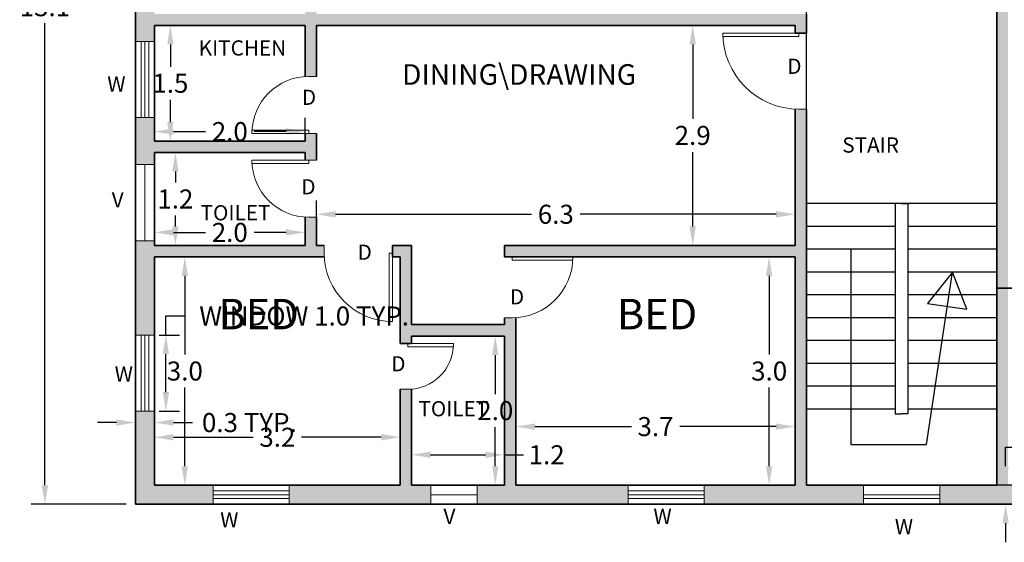
# Model space of a CAD drawing. Units: metres. Extents: x 6.2 to 29.4, y -2.1 to 16.8.
# Tile 1 of 3: x 6.2 to 19.2, y -2.1 to 4.8. Entities that reach past the tile are written whole.
import ezdxf

# ---------------------------------------------------------------- set-up
doc = ezdxf.new("R2010")
doc.units = ezdxf.units.M
doc.header["$MEASUREMENT"] = 0
doc.layers.get('0').update_dxf_attribs({"color": 2})
doc.layers.get('Defpoints').update_dxf_attribs({"color": 3})
for name, color, linetype, lineweight in [('A-ANNO-DIMS', 6, 'Continuous', 13), ('A-ANNO-TEXT', 7, 'Continuous', 18), ('A-AREA-IDEN', 3, 'Continuous', 18), ('A-DOOR', 3, 'Continuous', 18), ('A-FLOR-STRS', 1, 'Continuous', 25), ('A-GLAZ', 4, 'Continuous', 18), ('A-WALL', 7, 'Continuous', 35), ('A-WALL-PATT', 252, 'Continuous', 13)]:
    doc.layers.add(name, color=color, linetype=linetype, lineweight=lineweight)
doc.styles.get("Standard").update_dxf_attribs({"font": 'arial.ttf'})
doc.dimstyles.get("Standard").update_dxf_attribs({"dimtxt": 0.25, "dimasz": 0.25, "dimexe": 0.18, "dimexo": 0.0625, "dimgap": 0.09, "dimtad": 0, "dimtih": 1, "dimtoh": 1, "dimdec": 1, "dimzin": 0, "dimdsep": 46, "dimtxsty": 'Standard', "dimcen": 0.09, "dimadec": 0, "dimazin": 0, "dimtfac": 1, "dimtdec": 1, "dimtofl": 0, "dimtmove": 0, "dimatfit": 3, "dimfxl": 1, "dimtolj": 1, "dimtzin": 0, "dimarcsym": 0})

# ---------------------------------------------------------------- blocks, each defined once
blk = doc.blocks.new('*U2')
for p, q in [((-900, 0), (-900, 100)), ((0, 0), (0, 100))]:
    blk.add_line(p, q)
blk.add_lwpolyline([(0, 0), (0, -900), (-43.75, -900), (-43.75, 0)], close=True)
blk.add_arc((0, 0), 900, 180, 270)
blk = doc.blocks.new('*U3')
for p, q in [((0, 0), (0, -100)), ((600, 0), (600, -100))]:
    blk.add_line(p, q)
blk.add_lwpolyline([(0, 0), (0, 600), (43.75, 600), (43.75, 0)], close=True)
blk.add_arc((0, 0), 600, 0, 90)
blk = doc.blocks.new('*U4')
for p, q in [((-800, 0), (-800, 100)), ((0, 0), (0, 100))]:
    blk.add_line(p, q)
blk.add_lwpolyline([(0, 0), (0, -800), (-43.75, -800), (-43.75, 0)], close=True)
blk.add_arc((0, 0), 800, 180, 270)
blk = doc.blocks.new('*D5')
at = {"layer": 'A-ANNO-DIMS', "color": 0, "lineweight": -2, "transparency": 16777216}
for p, q in [((8.047, 1.673), (8.563, 1.673)), ((8.383, 1.423), (8.383, 0.391)), ((8.383, -1.077), (8.383, -0.045)), ((8.047, -1.327), (8.563, -1.327))]:
    blk.add_line(p, q, dxfattribs=at)
at = {"layer": 'A-ANNO-DIMS', "color": 0, "transparency": 16777216}
for points in [[(8.341, 1.423), (8.424, 1.423), (8.383, 1.673)], [(8.341, -1.077), (8.424, -1.077), (8.383, -1.327)]]:
    blk.add_solid(points, dxfattribs=at)
at = {"layer": 'Defpoints', "color": 0, "transparency": 16777216}
for p in [(7.984, 1.673), (7.984, -1.327), (8.383, -1.327)]:
    blk.add_point(p, dxfattribs=at)
at = {"layer": 'A-ANNO-DIMS', "color": 0, "transparency": 16777216, "insert": (8.383, 0.173), "char_height": 0.25, "attachment_point": 5}
blk.add_mtext('\\A1;3.0', dxfattribs=at)
blk = doc.blocks.new('*D6')
at = {"layer": 'A-ANNO-DIMS', "color": 0, "lineweight": -2, "transparency": 16777216}
for p, q in [((7.984, -1.264), (7.984, -0.517)), ((11.214, -1.264), (11.214, -0.517)), ((8.234, -0.697), (9.283, -0.697)), ((10.964, -0.697), (9.915, -0.697))]:
    blk.add_line(p, q, dxfattribs=at)
at = {"layer": 'A-ANNO-DIMS', "color": 0, "transparency": 16777216}
for points in [[(8.234, -0.655), (8.234, -0.739), (7.984, -0.697)], [(10.964, -0.655), (10.964, -0.739), (11.214, -0.697)]]:
    blk.add_solid(points, dxfattribs=at)
at = {"layer": 'Defpoints', "color": 0, "transparency": 16777216}
for p in [(11.214, -0.697), (7.984, -1.327), (11.214, -1.327)]:
    blk.add_point(p, dxfattribs=at)
at = {"layer": 'A-ANNO-DIMS', "color": 0, "transparency": 16777216, "insert": (9.599, -0.697), "char_height": 0.25, "attachment_point": 5}
blk.add_mtext('\\A1;3.2', dxfattribs=at)
blk = doc.blocks.new('*D7')
at = {"layer": 'A-ANNO-DIMS', "color": 0, "lineweight": -2, "transparency": 16777216}
for p, q in [((12.522, 0.633), (12.283, 0.633)), ((12.463, 0.383), (12.463, -0.129)), ((12.463, -1.077), (12.463, -0.565)), ((12.522, -1.327), (12.283, -1.327))]:
    blk.add_line(p, q, dxfattribs=at)
at = {"layer": 'A-ANNO-DIMS', "color": 0, "transparency": 16777216}
for points in [[(12.421, 0.383), (12.504, 0.383), (12.463, 0.633)], [(12.421, -1.077), (12.504, -1.077), (12.463, -1.327)]]:
    blk.add_solid(points, dxfattribs=at)
at = {"layer": 'Defpoints', "color": 0, "transparency": 16777216}
for p in [(12.584, 0.633), (12.463, -1.327), (12.584, -1.327)]:
    blk.add_point(p, dxfattribs=at)
at = {"layer": 'A-ANNO-DIMS', "color": 0, "transparency": 16777216, "insert": (12.463, -0.347), "char_height": 0.25, "attachment_point": 5}
blk.add_mtext('\\A1;2.0', dxfattribs=at)
blk = doc.blocks.new('*D8')
at = {"layer": 'A-ANNO-DIMS', "color": 0, "lineweight": -2, "transparency": 16777216}
for p, q in [((11.364, -1.264), (11.364, -0.747)), ((12.584, -1.264), (12.584, -0.747)), ((11.614, -0.927), (12.334, -0.927)), ((12.584, -0.927), (12.834, -0.927))]:
    blk.add_line(p, q, dxfattribs=at)
at = {"layer": 'A-ANNO-DIMS', "color": 0, "transparency": 16777216}
for points in [[(11.614, -0.886), (11.614, -0.969), (11.364, -0.927)], [(12.334, -0.886), (12.334, -0.969), (12.584, -0.927)]]:
    blk.add_solid(points, dxfattribs=at)
at = {"layer": 'Defpoints', "color": 0, "transparency": 16777216}
for p in [(12.584, -0.927), (11.364, -1.327), (12.584, -1.327)]:
    blk.add_point(p, dxfattribs=at)
at = {"layer": 'A-ANNO-DIMS', "color": 0, "transparency": 16777216, "insert": (13.139, -0.927), "char_height": 0.25, "attachment_point": 5}
blk.add_mtext('\\A1;1.2', dxfattribs=at)
blk = doc.blocks.new('*D9')
at = {"layer": 'A-ANNO-DIMS', "color": 0, "lineweight": -2, "transparency": 16777216}
for p, q in [((16.342, 1.673), (15.883, 1.673)), ((16.063, 1.423), (16.063, 0.391)), ((16.063, -1.077), (16.063, -0.045)), ((16.342, -1.327), (15.883, -1.327))]:
    blk.add_line(p, q, dxfattribs=at)
at = {"layer": 'A-ANNO-DIMS', "color": 0, "transparency": 16777216}
for points in [[(16.021, 1.423), (16.104, 1.423), (16.063, 1.673)], [(16.021, -1.077), (16.104, -1.077), (16.063, -1.327)]]:
    blk.add_solid(points, dxfattribs=at)
at = {"layer": 'Defpoints', "color": 0, "transparency": 16777216}
for p in [(16.404, 1.673), (16.063, -1.327), (16.404, -1.327)]:
    blk.add_point(p, dxfattribs=at)
at = {"layer": 'A-ANNO-DIMS', "color": 0, "transparency": 16777216, "insert": (16.063, 0.173), "char_height": 0.25, "attachment_point": 5}
blk.add_mtext('\\A1;3.0', dxfattribs=at)
blk = doc.blocks.new('*D10')
at = {"layer": 'A-ANNO-DIMS', "color": 0, "lineweight": -2, "transparency": 16777216}
for p, q in [((12.734, -1.264), (12.734, -0.377)), ((16.404, -1.264), (16.404, -0.377)), ((12.984, -0.557), (14.252, -0.557)), ((16.154, -0.557), (14.887, -0.557))]:
    blk.add_line(p, q, dxfattribs=at)
at = {"layer": 'A-ANNO-DIMS', "color": 0, "transparency": 16777216}
for points in [[(12.984, -0.516), (12.984, -0.599), (12.734, -0.557)], [(16.154, -0.516), (16.154, -0.599), (16.404, -0.557)]]:
    blk.add_solid(points, dxfattribs=at)
at = {"layer": 'Defpoints', "color": 0, "transparency": 16777216}
for p in [(16.404, -0.557), (12.734, -1.327), (16.404, -1.327)]:
    blk.add_point(p, dxfattribs=at)
at = {"layer": 'A-ANNO-DIMS', "color": 0, "transparency": 16777216, "insert": (14.569, -0.557), "char_height": 0.25, "attachment_point": 5}
blk.add_mtext('\\A1;3.7', dxfattribs=at)
blk = doc.blocks.new('*U17')
for p, q in [((-750, 0), (-750, -100)), ((0, 0), (0, -100))]:
    blk.add_line(p, q)
blk.add_lwpolyline([(0, 0), (0, 750), (-43.75, 750), (-43.75, 0)], close=True)
blk.add_arc((0, 0), 750, 90, 180)
blk = doc.blocks.new('*D18')
at = {"layer": 'A-ANNO-DIMS', "color": 0, "lineweight": -2, "transparency": 16777216}
for p, q in [((8.047, 4.713), (8.373, 4.713)), ((8.193, 4.463), (8.193, 4.171)), ((8.193, 3.443), (8.193, 3.735)), ((8.047, 3.193), (8.373, 3.193))]:
    blk.add_line(p, q, dxfattribs=at)
at = {"layer": 'A-ANNO-DIMS', "color": 0, "transparency": 16777216}
for points in [[(8.151, 4.463), (8.234, 4.463), (8.193, 4.713)], [(8.151, 3.443), (8.234, 3.443), (8.193, 3.193)]]:
    blk.add_solid(points, dxfattribs=at)
at = {"layer": 'Defpoints', "color": 0, "transparency": 16777216}
for p in [(7.984, 4.713), (7.984, 3.193), (8.193, 3.193)]:
    blk.add_point(p, dxfattribs=at)
at = {"layer": 'A-ANNO-DIMS', "color": 0, "transparency": 16777216, "insert": (8.193, 3.953), "char_height": 0.25, "attachment_point": 5}
blk.add_mtext('\\A1;1.5', dxfattribs=at)
blk = doc.blocks.new('*D19')
at = {"layer": 'A-ANNO-DIMS', "color": 0, "lineweight": -2, "transparency": 16777216}
for p, q in [((7.984, 3.256), (7.984, 3.498)), ((9.964, 3.256), (9.964, 3.498)), ((8.234, 3.318), (8.655, 3.318)), ((9.714, 3.318), (9.293, 3.318))]:
    blk.add_line(p, q, dxfattribs=at)
at = {"layer": 'A-ANNO-DIMS', "color": 0, "transparency": 16777216}
for points in [[(8.234, 3.36), (8.234, 3.277), (7.984, 3.318)], [(9.714, 3.36), (9.714, 3.277), (9.964, 3.318)]]:
    blk.add_solid(points, dxfattribs=at)
at = {"layer": 'Defpoints', "color": 0, "transparency": 16777216}
for p in [(7.984, 3.318), (7.984, 3.193), (9.964, 3.193)]:
    blk.add_point(p, dxfattribs=at)
at = {"layer": 'A-ANNO-DIMS', "color": 0, "transparency": 16777216, "insert": (8.974, 3.318), "char_height": 0.25, "attachment_point": 5}
blk.add_mtext('\\A1;2.0', dxfattribs=at)
blk = doc.blocks.new('*D20')
at = {"layer": 'A-ANNO-DIMS', "color": 0, "lineweight": -2, "transparency": 16777216}
for p, q in [((8.047, 3.043), (8.439, 3.043)), ((8.259, 2.793), (8.259, 2.649)), ((8.259, 2.073), (8.259, 2.218)), ((8.047, 1.823), (8.439, 1.823))]:
    blk.add_line(p, q, dxfattribs=at)
at = {"layer": 'A-ANNO-DIMS', "color": 0, "transparency": 16777216}
for points in [[(8.217, 2.793), (8.301, 2.793), (8.259, 3.043)], [(8.217, 2.073), (8.301, 2.073), (8.259, 1.823)]]:
    blk.add_solid(points, dxfattribs=at)
at = {"layer": 'Defpoints', "color": 0, "transparency": 16777216}
for p in [(7.984, 3.043), (7.984, 1.823), (8.259, 1.823)]:
    blk.add_point(p, dxfattribs=at)
at = {"layer": 'A-ANNO-DIMS', "color": 0, "transparency": 16777216, "insert": (8.259, 2.433), "char_height": 0.25, "attachment_point": 5}
blk.add_mtext('\\A1;1.2', dxfattribs=at)
blk = doc.blocks.new('*D21')
at = {"layer": 'A-ANNO-DIMS', "color": 0, "lineweight": -2, "transparency": 16777216}
for p, q in [((7.984, 1.886), (7.984, 2.174)), ((9.964, 1.886), (9.964, 2.174)), ((8.234, 1.994), (8.655, 1.994)), ((9.714, 1.994), (9.293, 1.994))]:
    blk.add_line(p, q, dxfattribs=at)
at = {"layer": 'A-ANNO-DIMS', "color": 0, "transparency": 16777216}
for points in [[(8.234, 2.036), (8.234, 1.952), (7.984, 1.994)], [(9.714, 2.036), (9.714, 1.952), (9.964, 1.994)]]:
    blk.add_solid(points, dxfattribs=at)
at = {"layer": 'Defpoints', "color": 0, "transparency": 16777216}
for p in [(7.984, 1.994), (7.984, 1.823), (9.964, 1.823)]:
    blk.add_point(p, dxfattribs=at)
at = {"layer": 'A-ANNO-DIMS', "color": 0, "transparency": 16777216, "insert": (8.974, 1.994), "char_height": 0.25, "attachment_point": 5}
blk.add_mtext('\\A1;2.0', dxfattribs=at)
blk = doc.blocks.new('*U22')
for p, q in [((0, 0), (0, -100)), ((-1000, 0), (-1000, -100))]:
    blk.add_line(p, q)
blk.add_lwpolyline([(0, 0), (0, 1000), (-43.75, 1000), (-43.75, 0)], close=True)
blk.add_arc((0, 0), 1000, 90, 180)
blk = doc.blocks.new('*D23')
at = {"layer": 'A-ANNO-DIMS', "color": 0, "lineweight": -2, "transparency": 16777216}
for p, q in [((14.995, 4.713), (14.878, 4.713)), ((15.058, 4.463), (15.058, 3.486)), ((15.058, 2.073), (15.058, 3.05)), ((14.995, 1.823), (14.878, 1.823))]:
    blk.add_line(p, q, dxfattribs=at)
at = {"layer": 'A-ANNO-DIMS', "color": 0, "transparency": 16777216}
for points in [[(15.016, 4.463), (15.1, 4.463), (15.058, 4.713)], [(15.016, 2.073), (15.1, 2.073), (15.058, 1.823)]]:
    blk.add_solid(points, dxfattribs=at)
at = {"layer": 'Defpoints', "color": 0, "transparency": 16777216}
for p in [(15.058, 4.713), (15.058, 1.823), (15.058, 1.823)]:
    blk.add_point(p, dxfattribs=at)
at = {"layer": 'A-ANNO-DIMS', "color": 0, "transparency": 16777216, "insert": (15.058, 3.268), "char_height": 0.25, "attachment_point": 5}
blk.add_mtext('\\A1;2.9', dxfattribs=at)
blk = doc.blocks.new('*D24')
at = {"layer": 'A-ANNO-DIMS', "color": 0, "lineweight": -2, "transparency": 16777216}
for p, q in [((10.114, 2.071), (10.114, 2.412)), ((16.404, 2.071), (16.404, 2.412)), ((10.364, 2.232), (12.941, 2.232)), ((16.154, 2.232), (13.577, 2.232))]:
    blk.add_line(p, q, dxfattribs=at)
at = {"layer": 'A-ANNO-DIMS', "color": 0, "transparency": 16777216}
for points in [[(10.364, 2.274), (10.364, 2.19), (10.114, 2.232)], [(16.154, 2.274), (16.154, 2.19), (16.404, 2.232)]]:
    blk.add_solid(points, dxfattribs=at)
at = {"layer": 'Defpoints', "color": 0, "transparency": 16777216}
for p in [(16.404, 2.232), (10.114, 2.008), (16.404, 2.008)]:
    blk.add_point(p, dxfattribs=at)
at = {"layer": 'A-ANNO-DIMS', "color": 0, "transparency": 16777216, "insert": (13.259, 2.232), "char_height": 0.25, "attachment_point": 5}
blk.add_mtext('\\A1;6.3', dxfattribs=at)
blk = doc.blocks.new('*D60')
at = {"layer": 'A-ANNO-DIMS', "color": 0, "lineweight": -2, "transparency": 16777216}
for p, q in [((7.611, 11.494), (6.364, 11.494)), ((6.544, 11.244), (6.544, 5.176)), ((6.544, -1.327), (6.544, 4.741)), ((7.611, -1.577), (6.364, -1.577))]:
    blk.add_line(p, q, dxfattribs=at)
at = {"layer": 'A-ANNO-DIMS', "color": 0, "transparency": 16777216}
for points in [[(6.502, 11.244), (6.586, 11.244), (6.544, 11.494)], [(6.502, -1.327), (6.586, -1.327), (6.544, -1.577)]]:
    blk.add_solid(points, dxfattribs=at)
at = {"layer": 'Defpoints', "color": 0, "transparency": 16777216}
for p in [(7.674, 11.494), (6.544, -1.577), (7.674, -1.577)]:
    blk.add_point(p, dxfattribs=at)
at = {"layer": 'A-ANNO-DIMS', "color": 0, "transparency": 16777216, "insert": (6.544, 4.959), "char_height": 0.25, "attachment_point": 5}
blk.add_mtext('\\A1;13.1', dxfattribs=at)
blk = doc.blocks.new('WIN-1000')
for p, q in [((0.075, 1), (0.075, 0)), ((0.125, 1), (0.125, 0)), ((0.175, 1), (0.175, 0))]:
    blk.add_line(p, q)
blk.add_lwpolyline([(0, 1), (0.25, 1), (0.25, 0), (0, 0)], close=True)
blk = doc.blocks.new('VENT-1000')
blk.add_line((0.125, 1), (0.125, 0))
blk.add_lwpolyline([(0, 1), (0.25, 1), (0.25, 0), (0, 0)], close=True)
blk = doc.blocks.new('*D65')
at = {"layer": 'A-ANNO-DIMS', "color": 0, "lineweight": -2, "transparency": 16777216}
for p, q in [((8.134, 0.646), (8.134, 0.896)), ((8.134, 0.896), (8.384, 0.896)), ((8.047, 0.646), (8.314, 0.646)), ((8.134, -0.104), (8.134, 0.396)), ((8.047, -0.354), (8.314, -0.354))]:
    blk.add_line(p, q, dxfattribs=at)
at = {"layer": 'A-ANNO-DIMS', "color": 0, "transparency": 16777216}
for points in [[(8.092, 0.396), (8.176, 0.396), (8.134, 0.646)], [(8.092, -0.104), (8.176, -0.104), (8.134, -0.354)]]:
    blk.add_solid(points, dxfattribs=at)
at = {"layer": 'Defpoints', "color": 0, "transparency": 16777216}
for p in [(7.984, 0.646), (8.134, 0.646), (7.984, -0.354)]:
    blk.add_point(p, dxfattribs=at)
at = {"layer": 'A-ANNO-DIMS', "color": 0, "transparency": 16777216, "insert": (9.951, 0.896), "char_height": 0.25, "attachment_point": 5}
blk.add_mtext('\\A1;WINDOW 1.0 TYP.', dxfattribs=at)
blk = doc.blocks.new('*D66')
at = {"layer": 'A-ANNO-DIMS', "color": 0, "lineweight": -2, "transparency": 16777216}
for p, q in [((7.484, -0.504), (7.234, -0.504)), ((7.734, -0.416), (7.734, -0.684)), ((7.984, -0.416), (7.984, -0.684)), ((8.234, -0.504), (8.484, -0.504))]:
    blk.add_line(p, q, dxfattribs=at)
at = {"layer": 'A-ANNO-DIMS', "color": 0, "transparency": 16777216}
for points in [[(7.484, -0.462), (7.484, -0.545), (7.734, -0.504)], [(8.234, -0.462), (8.234, -0.545), (7.984, -0.504)]]:
    blk.add_solid(points, dxfattribs=at)
at = {"layer": 'Defpoints', "color": 0, "transparency": 16777216}
for p in [(7.734, -0.354), (7.984, -0.354), (7.984, -0.504)]:
    blk.add_point(p, dxfattribs=at)
at = {"layer": 'A-ANNO-DIMS', "color": 0, "transparency": 16777216, "insert": (9.231, -0.504), "char_height": 0.25, "attachment_point": 5}
blk.add_mtext('\\A1;0.3 TYP.', dxfattribs=at)
blk = doc.blocks.new('*D70')
at = {"layer": 'A-ANNO-DIMS', "color": 0, "lineweight": -2, "transparency": 16777216}
for p, q in [((19.17, -1.077), (19.17, -0.827)), ((19.17, -0.827), (19.42, -0.827)), ((19.258, -1.327), (18.99, -1.327)), ((19.258, -1.577), (18.99, -1.577)), ((19.17, -1.827), (19.17, -2.077))]:
    blk.add_line(p, q, dxfattribs=at)
at = {"layer": 'A-ANNO-DIMS', "color": 0, "transparency": 16777216}
for points in [[(19.129, -1.077), (19.212, -1.077), (19.17, -1.327)], [(19.129, -1.827), (19.212, -1.827), (19.17, -1.577)]]:
    blk.add_solid(points, dxfattribs=at)
at = {"layer": 'Defpoints', "color": 0, "transparency": 16777216}
for p in [(19.17, -1.327), (19.32, -1.327), (19.32, -1.577)]:
    blk.add_point(p, dxfattribs=at)
at = {"layer": 'A-ANNO-DIMS', "color": 0, "transparency": 16777216, "insert": (20.167, -0.827), "char_height": 0.25, "attachment_point": 5}
blk.add_mtext('\\A1;0.3 TYP.', dxfattribs=at)
blk = doc.blocks.new('*D71')
at = {"layer": 'A-ANNO-DIMS', "color": 0, "lineweight": -2, "transparency": 16777216}
for p, q in [((16.554, 2.436), (16.554, 15.849)), ((19.054, 2.436), (19.054, 15.849)), ((16.804, 15.669), (17.483, 15.669)), ((18.804, 15.669), (18.125, 15.669))]:
    blk.add_line(p, q, dxfattribs=at)
at = {"layer": 'A-ANNO-DIMS', "color": 0, "transparency": 16777216}
for points in [[(16.804, 15.71), (16.804, 15.627), (16.554, 15.669)], [(18.804, 15.71), (18.804, 15.627), (19.054, 15.669)]]:
    blk.add_solid(points, dxfattribs=at)
at = {"layer": 'Defpoints', "color": 0, "transparency": 16777216}
for p in [(19.054, 15.669), (16.554, 2.373), (19.054, 2.373)]:
    blk.add_point(p, dxfattribs=at)
at = {"layer": 'A-ANNO-DIMS', "color": 0, "transparency": 16777216, "insert": (17.804, 15.669), "char_height": 0.25, "attachment_point": 5}
blk.add_mtext('\\A1;2.5', dxfattribs=at)

msp = doc.modelspace()

# ---------------------------------------------------------------- hatches: boundary and pattern name
at = {"layer": 'A-WALL-PATT'}
h = msp.add_hatch(dxfattribs=at)
h.set_pattern_fill('BRICK', color=256, scale=0.3)
h.paths.add_polyline_path([(26.024, -0.354), (25.774, -0.354), (25.774, -1.327), (24.478, -1.327), (24.478, -1.577), (26.024, -1.577)])
h.paths.add_polyline_path([(26.024, 2.199), (25.774, 2.199), (25.774, 2.123), (24.325, 2.123, -0.063254), (24.344, 1.973), (24.344, 1.873), (25.774, 1.873), (25.774, 0.646), (26.024, 0.646)])
h.paths.add_polyline_path([(26.624, 4.802), (26.374, 4.802), (26.374, 3.493), (23.373, 3.493, -0.013897), (23.374, 3.443), (23.374, 3.343), (23.494, 3.343), (23.494, 2.123), (23.344, 2.123), (23.344, 2.023, -0.03766), (23.333, 1.873), (23.744, 1.873), (23.744, 1.973), (23.744, 2.123), (23.644, 2.123), (23.644, 3.343), (25.774, 3.343), (25.774, 3.199), (26.024, 3.199), (26.024, 3.343), (26.624, 3.343)])
h.paths.add_polyline_path([(26.624, 6.775), (26.374, 6.775), (26.374, 6.693), (24.244, 6.693), (24.244, 7.065, -0.016681), (24.194, 7.063), (24.094, 7.063), (24.094, 6.693), (19.054, 6.693), (19.054, 6.443), (19.154, 6.443), (19.204, 6.443), (19.204, 6.543), (22.224, 6.543), (22.224, 3.343), (22.474, 3.343), (22.474, 3.443), (22.474, 3.493), (22.374, 3.493), (22.374, 6.543), (26.374, 6.543), (26.374, 5.802), (26.624, 5.802)])
h.paths.add_polyline_path([(26.624, 8.282), (26.374, 8.282), (26.374, 8.063), (24.244, 8.063), (24.244, 8.163), (24.194, 8.163), (24.094, 8.163), (24.094, 7.813), (24.194, 7.813), (24.244, 7.813), (24.244, 7.913), (26.374, 7.913), (26.374, 7.775), (26.624, 7.775)])
h.paths.add_polyline_path([(26.624, 9.85), (26.374, 9.85), (26.374, 9.733), (24.244, 9.733), (24.244, 10.953), (24.344, 10.953), (24.344, 11.003), (24.344, 11.103), (22.814, 11.103), (22.814, 10.953), (24.094, 10.953), (24.094, 8.913), (24.194, 8.913, -0.016681), (24.244, 8.911), (24.244, 9.583), (26.374, 9.583), (26.374, 9.282), (26.624, 9.282)])
h.paths.add_polyline_path([(26.624, 14.583), (24.36, 14.583), (24.36, 14.333), (25.424, 14.333), (25.424, 11.953), (25.524, 11.953, -0.016681), (25.574, 11.951), (25.574, 14.333), (26.374, 14.333), (26.374, 11.103), (25.574, 11.103), (25.574, 11.203), (25.524, 11.203), (25.424, 11.203), (25.424, 11.103), (25.094, 11.103), (25.094, 11.003, -0.016681), (25.092, 10.953), (26.374, 10.953), (26.374, 10.85), (26.624, 10.85)])
h.paths.add_polyline_path([(23.36, 14.583), (21.664, 14.583), (21.664, 13.153), (20.023, 13.153), (20.023, 12.903), (21.664, 12.903), (21.664, 10.568, -0.050382), (21.814, 10.583), (21.914, 10.583), (21.914, 10.953), (22.014, 10.953), (22.014, 11.053), (22.014, 11.103), (21.914, 11.103), (21.914, 14.333), (23.36, 14.333)])
h.paths.add_polyline_path([(19.023, 13.153), (17.234, 13.153), (17.234, 12.453), (15.201, 12.453), (15.201, 12.203), (17.234, 12.203), (17.234, 8.643), (17.234, 6.543), (17.484, 6.543), (17.484, 6.643), (17.484, 6.693), (17.384, 6.693), (17.384, 9.683), (21.914, 9.683), (21.914, 9.833), (21.814, 9.833), (21.064, 9.833), (17.384, 9.833), (17.384, 12.903), (19.023, 12.903)])
h.paths.add_polyline_path([(14.201, 12.453), (12.964, 12.453), (12.964, 11.878), (12.801, 11.878), (12.801, 11.628), (12.964, 11.628), (12.964, 9.628), (11.744, 9.628), (11.744, 9.728), (11.694, 9.728), (11.594, 9.728), (11.594, 9.236, -0.016681), (11.644, 9.238), (11.744, 9.238), (11.744, 9.478), (12.964, 9.478), (12.964, 8.493), (13.214, 8.493), (13.214, 8.593), (13.214, 8.643), (13.114, 8.643), (13.114, 12.203), (14.201, 12.203)])
h.paths.add_polyline_path([(11.801, 11.878), (11.594, 11.878), (11.594, 11.494), (8.294, 11.494), (8.294, 10.872), (8.394, 10.872), (8.394, 11.378), (11.594, 11.378), (11.594, 10.478), (11.694, 10.478, -0.016681), (11.744, 10.476), (11.744, 11.628), (11.801, 11.628)])
h.paths.add_polyline_path([(8.394, 9.872), (8.294, 9.872), (8.294, 9.088), (8.394, 9.088)])
h.paths.add_polyline_path([(7.984, 7.122), (7.734, 7.122), (7.734, 6.491), (7.984, 6.491), (7.984, 6.658), (9.964, 6.658), (10.014, 6.658), (10.114, 6.658), (10.114, 6.808), (10.014, 6.808), (9.414, 6.808), (7.984, 6.808)])
h.paths.add_polyline_path([(7.984, 5.491), (7.734, 5.491), (7.734, 4.503), (7.984, 4.503), (7.984, 4.713), (9.964, 4.713), (9.964, 4.041, -0.016681), (10.014, 4.043), (10.114, 4.043), (10.114, 4.713), (16.404, 4.713), (16.404, 4.613), (16.454, 4.613), (16.554, 4.613), (16.554, 4.863), (10.114, 4.863), (10.114, 6.058), (10.014, 6.058, -0.020861), (9.964, 6.06), (9.964, 4.863), (7.984, 4.863)])
h.paths.add_polyline_path([(10.114, 3.293), (10.014, 3.293), (9.964, 3.293), (9.964, 3.193), (7.984, 3.193), (7.984, 3.503), (7.734, 3.503), (7.734, 2.884), (7.984, 2.884), (7.984, 3.043), (9.964, 3.043), (9.964, 2.943), (10.014, 2.943), (10.114, 2.943)])
h.paths.add_polyline_path([(7.984, 1.673), (10.216, 1.673, -0.013897), (10.214, 1.723), (10.214, 1.823), (10.114, 1.823), (10.114, 2.193), (10.014, 2.193, -0.016681), (9.964, 2.195), (9.964, 1.823), (7.984, 1.823), (7.984, 1.884), (7.734, 1.884), (7.734, 0.646), (7.984, 0.646)])
h.paths.add_polyline_path([(8.755, -1.327), (7.984, -1.327), (7.984, -0.354), (7.734, -0.354), (7.734, -1.577), (8.755, -1.577)])
h.paths.add_polyline_path([(11.615, -1.327), (11.364, -1.327), (11.364, -0.065, -0.020861), (11.314, -0.067), (11.214, -0.067), (11.214, -1.327), (9.755, -1.327), (9.755, -1.577), (11.615, -1.577)])
h.paths.add_polyline_path([(14.209, -1.327), (12.734, -1.327), (12.734, 0.875, -0.015636), (12.684, 0.873), (12.584, 0.873), (12.584, 0.783), (11.364, 0.783), (11.364, 1.823), (11.114, 1.823), (11.114, 1.723), (11.114, 1.673), (11.214, 1.673), (11.214, 0.533), (11.314, 0.533), (11.364, 0.533), (11.364, 0.633), (12.584, 0.633), (12.584, -1.327), (12.227, -1.327), (12.227, -1.577), (14.209, -1.577)])
h.paths.add_polyline_path([(17.304, -1.327), (16.554, -1.327), (16.554, 3.613), (16.454, 3.613, -0.012506), (16.404, 3.614), (16.404, 1.823), (12.584, 1.823), (12.584, 1.673), (12.684, 1.673), (13.484, 1.673), (16.404, 1.673), (16.404, -1.327), (15.209, -1.327), (15.209, -1.577), (17.304, -1.577)])
h.paths.add_polyline_path([(19.32, -1.327), (19.204, -1.327), (19.204, 1.263), (19.054, 1.263), (19.054, -1.327), (18.304, -1.327), (18.304, -1.577), (19.32, -1.577)])
h.paths.add_polyline_path([(23.478, -1.327), (22.244, -1.327), (22.244, 1.873), (22.344, 1.873), (22.344, 2.023), (22.344, 2.123), (22.094, 2.123), (22.094, 1.263), (21.374, 1.263), (21.374, 1.163, -0.016681), (21.372, 1.113), (22.094, 1.113), (22.094, -1.327), (21.86, -1.327), (21.86, -1.577), (23.478, -1.577)])
h.paths.add_polyline_path([(19.204, 5.444, -0.012506), (19.154, 5.443), (19.054, 5.443), (19.054, 1.263), (19.204, 1.263)])
h.paths.add_polyline_path([(19.054, 6.693), (18.483, 6.693, -0.012506), (18.484, 6.643), (18.484, 6.543), (19.054, 6.543)], flags=17)
h.paths.add_polyline_path([(11.744, 8.488), (7.674, 8.488), (7.674, 8.338), (7.734, 8.338), (7.734, 8.122), (7.984, 8.122), (7.984, 8.338), (9.964, 8.338), (9.964, 7.406, -0.020861), (10.014, 7.408), (10.114, 7.408), (10.114, 8.338), (11.744, 8.338)])
h.paths.add_polyline_path([(15.131, 11.42), (16.48, 11.42), (16.48, 12.245), (15.131, 12.245)], flags=9)
h.paths.add_polyline_path([(8.62, 7.608), (9.947, 7.608), (9.947, 8.021), (8.62, 8.021)], flags=24)

# ---------------------------------------------------------------- linework, layer by layer
at = {"layer": 'A-DOOR'}
msp.add_line((9.964, 3.293), (9.264, 3.293), dxfattribs=at)
at = {"layer": 'A-FLOR-STRS'}
for p, q in [((19.054, 2.373), (16.554, 2.373)), ((17.721, 2.073), (16.554, 2.073)), ((19.054, 2.073), (17.887, 2.073)), ((17.721, 1.773), (16.554, 1.773)), ((19.054, 1.773), (17.887, 1.773)), ((17.721, 1.473), (16.554, 1.473)), ((19.054, 1.473), (17.887, 1.473)), ((17.721, 1.173), (16.554, 1.173)), ((19.054, 1.173), (17.887, 1.173)), ((17.721, 0.873), (16.554, 0.873)), ((19.054, 0.873), (17.887, 0.873)), ((17.721, 0.573), (16.554, 0.573)), ((19.054, 0.573), (17.887, 0.573)), ((17.721, 0.273), (16.554, 0.273)), ((19.054, 0.273), (17.887, 0.273)), ((17.721, -0.027), (16.554, -0.027)), ((19.054, -0.027), (17.887, -0.027)), ((17.721, -0.327), (16.554, -0.327)), ((19.054, -0.327), (17.887, -0.327))]:
    msp.add_line(p, q, dxfattribs=at)
for points in [[(17.804, 2.373), (17.721, 2.373), (17.721, -0.389), (17.804, -0.389)], [(17.804, 2.373), (17.887, 2.373), (17.887, -0.389), (17.804, -0.389)], [(17.138, 1.773), (17.138, -0.792), (18.13, -0.792), (18.471, 1.473)]]:
    msp.add_lwpolyline(points, dxfattribs=at)
msp.add_lwpolyline([(18.471, 1.473), (18.143, 1.062), (18.663, 0.984)], close=True, dxfattribs=at)
at = {"layer": 'A-GLAZ'}
for p, q in [((17.304, -1.327), (18.304, -1.327)), ((11.615, -1.452), (12.227, -1.452)), ((17.304, -1.452), (18.304, -1.452)), ((17.304, -1.502), (18.304, -1.502))]:
    msp.add_line(p, q, dxfattribs=at)
for points in [[(11.615, -1.327), (12.227, -1.327), (12.227, -1.577), (11.615, -1.577)], [(17.304, -1.327), (18.304, -1.327), (18.304, -1.577), (17.304, -1.577)]]:
    msp.add_lwpolyline(points, close=True, dxfattribs=at)
at = {"layer": 'A-WALL'}
for p, q in [((7.734, -1.577), (7.734, 8.338)), ((19.054, -1.327), (19.054, 5.443)), ((16.554, 4.613), (16.554, 4.863)), ((7.984, 3.193), (7.984, 4.713)), ((9.964, 4.713), (7.984, 4.713)), ((9.964, 4.041), (9.964, 4.713)), ((16.404, 4.713), (10.114, 4.713)), ((10.114, 4.043), (10.114, 4.713)), ((16.404, 4.613), (16.404, 4.713)), ((16.404, 4.613), (16.554, 4.613)), ((16.404, 1.823), (16.404, 3.614)), ((16.554, -1.327), (16.554, 3.613)), ((9.964, 3.193), (9.964, 3.293)), ((10.114, 2.943), (10.114, 3.293)), ((9.964, 3.193), (7.984, 3.193)), ((7.984, 1.823), (7.984, 3.043)), ((9.964, 3.043), (7.984, 3.043)), ((9.964, 2.943), (9.964, 3.043)), ((9.964, 1.823), (9.964, 2.195)), ((10.114, 1.823), (10.114, 2.193)), ((9.964, 1.823), (7.984, 1.823)), ((10.214, 1.823), (10.114, 1.823)), ((11.364, 1.823), (11.114, 1.823)), ((11.114, 1.673), (11.114, 1.823)), ((11.364, 0.783), (11.364, 1.823)), ((16.404, 1.823), (12.584, 1.823)), ((12.584, 1.673), (12.584, 1.823)), ((7.984, -1.327), (7.984, 1.673)), ((10.216, 1.673), (7.984, 1.673)), ((11.214, 1.673), (11.114, 1.673)), ((11.214, 0.533), (11.214, 1.673)), ((16.404, 1.673), (12.584, 1.673)), ((16.404, -1.327), (16.404, 1.673)), ((19.624, 1.263), (19.054, 1.263)), ((12.584, 0.783), (11.364, 0.783)), ((12.584, 0.783), (12.584, 0.873)), ((12.734, -1.327), (12.734, 0.875)), ((11.364, 0.533), (11.214, 0.533)), ((12.584, 0.633), (11.364, 0.633)), ((11.364, 0.533), (11.364, 0.633)), ((12.584, -1.327), (12.584, 0.633)), ((11.214, -1.327), (11.214, -0.067)), ((11.364, -1.327), (11.364, -0.065)), ((11.214, -1.327), (7.984, -1.327)), ((12.584, -1.327), (11.364, -1.327)), ((16.404, -1.327), (12.734, -1.327)), ((19.054, -1.327), (16.554, -1.327)), ((26.024, -1.577), (7.734, -1.577))]:
    msp.add_line(p, q, dxfattribs=at)

# ---------------------------------------------------------------- block references
at = {"layer": 'A-DOOR', "yscale": 0.001, "zscale": 0.001}
for name, p, xscale, rotation in [('*U22', (16.454, 4.613), 0.001, 90), ('*U17', (10.014, 3.293), -0.001, 90), ('*U17', (10.014, 2.943), 0.001, 90), ('*U4', (12.684, 1.673), 0.001, 90), ('*U3', (11.314, 0.533), 0.001, 270)]:
    msp.add_blockref(name, p, dxfattribs=dict(at, xscale=xscale, rotation=rotation))
at = {"layer": 'A-DOOR', "xscale": 0.001, "yscale": 0.001, "zscale": 0.001}
msp.add_blockref('*U2', (11.114, 1.723), dxfattribs=at)
at = {"layer": 'A-GLAZ'}
for name, p in [('WIN-1000', (7.733, 3.503)), ('VENT-1000', (7.731, 1.884)), ('WIN-1000', (7.734, -0.354))]:
    msp.add_blockref(name, p, dxfattribs=at)
at = {"layer": 'A-GLAZ', "extrusion": (0, 0, -1), "zscale": -1, "rotation": 270.0000000000002}
for p in [(-9.755, -1.327), (-15.209, -1.327)]:
    msp.add_blockref('WIN-1000', p, dxfattribs=at)

# ---------------------------------------------------------------- texts
at = {"layer": 'A-ANNO-TEXT', "char_height": 0.2, "attachment_point": 1}
for s, insert in [('D ', (16.301, 4.277)), ('W ', (7.364, 4.043)), ('D ', (9.921, 3.869)), ('D ', (9.914, 2.693)), ('V ', (7.422, 2.522)), ('D ', (10.654, 1.834)), ('D ', (12.655, 1.248)), ('D ', (11.096, 0.368)), ('W ', (7.461, 0.233)), ('W ', (8.848, -1.682)), ('V ', (11.782, -1.636)), ('W ', (14.542, -1.635)), ('W ', (17.715, -1.771))]:
    msp.add_mtext_dynamic_manual_height_columns(s, width=0.50508, gutter_width=1, heights=[0], dxfattribs=dict(at, insert=insert))
at = {"layer": 'A-AREA-IDEN', "attachment_point": 1}
for s, width, gutter_width, insert, char_height in [('KITCHEN', 0.72932, 1, (8.565, 4.517), 0.2), ('DINING\\\\DRAWING', 2.52682, 1.356, (11.238, 4.204), 0.27123), ('STAIR', 0.82722, 1, (17.024, 3.242), 0.2), ('TOILET', 1.14866, 1, (8.59, 2.352), 0.2), ('BED', 1.14866, 1, (8.825, 1.121), 0.4), ('BED', 1.14866, 1, (14.062, 1.121), 0.4), ('TOILET', 1.14866, 1, (11.453, -0.222), 0.2)]:
    msp.add_mtext_dynamic_manual_height_columns(s, width=width, gutter_width=gutter_width, heights=[0], dxfattribs=dict(at, insert=insert, char_height=char_height))

# ---------------------------------------------------------------- dimensions: what is measured, and where the dimension line sits
at = {"layer": 'A-ANNO-DIMS'}
for base, p1, p2, override, picture, middle in [((19.054, 15.669), (16.554, 2.373), (19.054, 2.373), {"dimdec": 1, "dimlfac": 1, "dimrnd": 0, "dimzin": 0, "dimdsep": 46, "dimlunit": 2}, '*D71', (17.804, 15.669)), ((7.984, 3.318), (9.964, 3.193), (7.984, 3.193), {"dimclrd": 0, "dimclre": 0, "dimclrt": 0}, '*D19', (8.974, 3.318)), ((16.404, 2.232), (10.114, 2.008), (16.404, 2.008), {"dimclrd": 0, "dimclre": 0, "dimclrt": 0}, '*D24', (13.259, 2.232)), ((7.984, 1.994), (9.964, 1.823), (7.984, 1.823), {"dimclrd": 0, "dimclre": 0, "dimclrt": 0}, '*D21', (8.974, 1.994)), ((16.404, -0.557), (12.734, -1.327), (16.404, -1.327), {"dimclrd": 0, "dimclre": 0, "dimclrt": 0}, '*D10', (14.569, -0.557)), ((11.214, -0.697), (7.984, -1.327), (11.214, -1.327), {"dimclrd": 0, "dimclre": 0, "dimclrt": 0}, '*D6', (9.599, -0.697)), ((12.584, -0.927), (11.364, -1.327), (12.584, -1.327), {"dimclrd": 0, "dimclre": 0, "dimclrt": 0}, '*D8', (13.139, -0.927))]:
    dim = msp.add_linear_dim(base=base, p1=p1, p2=p2, dimstyle='Standard', override=override, dxfattribs=at)
    dim.commit()
    dim.dimension.update_dxf_attribs({"geometry": picture, "text_midpoint": middle})
for base, p1, p2, picture, middle in [((6.544, -1.577), (7.674, 11.494), (7.674, -1.577), '*D60', (6.544, 4.959)), ((8.193, 3.193), (7.984, 4.713), (7.984, 3.193), '*D18', (8.193, 3.953)), ((15.058, 1.823), (15.058, 4.713), (15.058, 1.823), '*D23', (15.058, 3.268)), ((8.259, 1.823), (7.984, 3.043), (7.984, 1.823), '*D20', (8.259, 2.433)), ((16.063, -1.327), (16.404, 1.673), (16.404, -1.327), '*D9', (16.063, 0.173)), ((12.463, -1.327), (12.584, 0.633), (12.584, -1.327), '*D7', (12.463, -0.347))]:
    dim = msp.add_linear_dim(base=base, p1=p1, p2=p2, angle=90, dimstyle='Standard', override={"dimclrd": 0, "dimclre": 0, "dimclrt": 0}, dxfattribs=at)
    dim.commit()
    dim.dimension.update_dxf_attribs({"geometry": picture, "text_midpoint": middle})
dim = msp.add_linear_dim(base=(8.383, -1.327), p1=(7.984, 1.673), p2=(7.984, -1.327), angle=90, dimstyle='Standard', override={"dimclrd": 0, "dimclre": 0, "dimclrt": 0}, dxfattribs=at)
dim.commit()
dim.dimension.update_dxf_attribs({"geometry": '*D5', "text_midpoint": (8.383, 0.173), "dimtype": 160})
for base, p1, p2, text, picture, middle in [((8.134, 0.646), (7.984, -0.354), (7.984, 0.646), 'WINDOW <> TYP.', '*D65', (9.951, 0.896)), ((19.170330791, -1.326870002), (19.320330791, -1.576870002), (19.320330791, -1.326870002), '<> TYP.', '*D70', (20.167305552, -0.826870002))]:
    dim = msp.add_linear_dim(base=base, p1=p1, p2=p2, angle=90, text=text, dimstyle='Standard', override={"dimdec": 1, "dimlfac": 1, "dimrnd": 0, "dimzin": 0, "dimdsep": 46, "dimlunit": 2}, dxfattribs=at)
    dim.commit()
    dim.dimension.update_dxf_attribs({"geometry": picture, "text_midpoint": middle})
dim = msp.add_linear_dim(base=(7.984114785, -0.503757433), p1=(7.734114785, -0.353757433), p2=(7.984114785, -0.353757433), text='<> TYP.', dimstyle='Standard', override={"dimdec": 1, "dimlfac": 1, "dimrnd": 0, "dimzin": 0, "dimdsep": 46, "dimlunit": 2}, dxfattribs=at)
dim.commit()
dim.dimension.update_dxf_attribs({"geometry": '*D66', "text_midpoint": (9.231089547, -0.503757433)})

doc.saveas('drawing.dxf')
